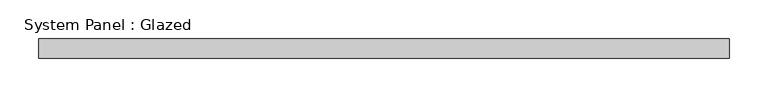
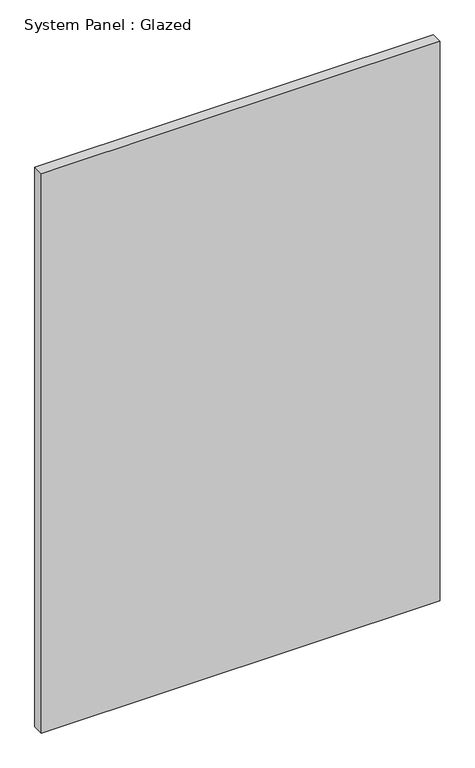
"""IFC4 building model written with IfcOpenShell, lengths in millimetres: plate geometry, System Panel : Glazed."""

from ifc_helpers import new_model, si_unit, origin, origin_with_axes, place, context, project, spatial, polyline, outline, extrude, source, transform, mapped, element, save


def system_panel_glazed_593bec76(model_context):
    return source(origin(), model_context, "Body", "SweptSolid", [
        extrude(outline(polyline([(447.675, 19.05), (-447.675, 19.05), (-447.675, 44.45), (447.675, 44.45), (447.675, 19.05)])), origin_with_axes(), (0.0, 0.0, 1.0), 1327.3964565),
    ])


if __name__ == "__main__":
    model = new_model("IFC4")
    model_context = context("Model", 3, world=origin())
    ifc_project = project(units=[si_unit("LENGTHUNIT", "METRE", prefix="MILLI")], contexts=[model_context])
    site = spatial("IfcSite", under=ifc_project)
    building = spatial("IfcBuilding", under=site)
    placement = place(None, origin())
    system_panel_glazed_shape = system_panel_glazed_593bec76(model_context)
    element("IfcPlate", 1, ObjectType="System Panel : Glazed", at=placement, inside=building, context=model_context, shape_type="MappedRepresentation", body=[
        mapped(system_panel_glazed_shape, transform((0.0, 0.0, 0.0), x_axis=(1.0, 0.0, 0.0), y_axis=(0.0, 1.0, 0.0), z_axis=(0.0, 0.0, 1.0))),
    ])
    save(model, "model.ifc")

# Revit data of these elements
# Type "System Panel : Glazed"
#   Construction Type Id = "GSP4R"
#   Analytic Construction = "1/8 in Pilkington single glazing"
#   Visual Light Transmittance = 0.9
#   Solar Heat Gain Coefficient = 0.86
#   Heat Transfer Coefficient (U) = 1.18115 BTU/(h·ft²·°F)
#   Define Thermal Properties by = 1
# Element 1 (IfcPlate, "System Panel : Glazed")
#   Materials on its faces: "Glass"
# Materials
#   "Glass": class "Glass", colour RGB 0 128 192, transparency 0.75, Description = "Soda Lime Glass", Cost = 0
